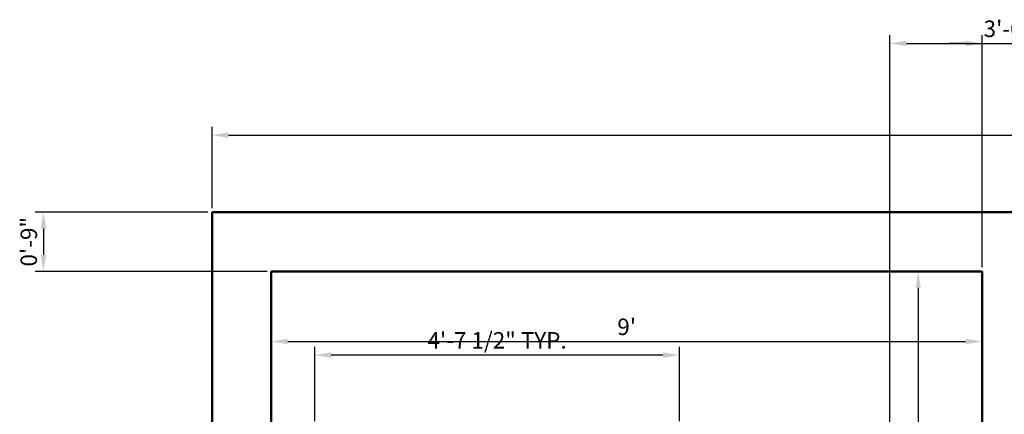
# Model space of a CAD drawing. Units: inches. Extents: x 2385 to 2740, y 1752 to 2305.
# Tile 10 of 15: x 2385 to 2535, y 2245 to 2305. Entities that reach past the tile are written whole.
import ezdxf

# ---------------------------------------------------------------- set-up
doc = ezdxf.new("R2010")
doc.units = ezdxf.units.IN
doc.layers.add('A-ANNO-DIMS', color=2, linetype='Continuous', lineweight=18)
doc.layers.add('A-WALL', color=7, linetype='Continuous', lineweight=50)
doc.styles.get("Standard").update_dxf_attribs({"font": 'arial.ttf'})
doc.dimstyles.new('Copy of ISO-25', dxfattribs={"dimtxt": 2.5, "dimasz": 2.5, "dimexe": 1.25, "dimexo": 0.625, "dimtad": 1, "dimdec": 1, "dimlunit": 4, "dimtxsty": 'Standard', "dimcen": 2.5, "dimadec": 0, "dimazin": 0, "dimtfac": 1, "dimtdec": 1, "dimtmove": 0, "dimatfit": 3, "dimfxl": 1, "dimarcsym": 0})

# ---------------------------------------------------------------- blocks, each defined once
blk = doc.blocks.new('*D6')
at = {"layer": 'A-ANNO-DIMS', "color": 0, "lineweight": -2, "transparency": 16777216}
for p, q in [((2423.25, 2266.34), (2423.25, 2255.07)), ((2531.25, 2266.34), (2531.25, 2255.07)), ((2425.75, 2256.32), (2528.75, 2256.32))]:
    blk.add_line(p, q, dxfattribs=at)
at = {"layer": 'A-ANNO-DIMS', "color": 0, "transparency": 16777216}
for points in [[(2425.75, 2256.74), (2425.75, 2255.91), (2423.25, 2256.32)], [(2528.75, 2256.74), (2528.75, 2255.91), (2531.25, 2256.32)]]:
    blk.add_solid(points, dxfattribs=at)
at = {"layer": 'Defpoints', "color": 0, "transparency": 16777216}
for p in [(2423.25, 2266.97), (2531.25, 2266.97), (2531.25, 2256.32)]:
    blk.add_point(p, dxfattribs=at)
at = {"layer": 'A-ANNO-DIMS', "color": 0, "transparency": 16777216, "insert": (2477.25, 2258.23), "char_height": 2.5, "attachment_point": 5}
blk.add_mtext("9'", dxfattribs=at)
blk = doc.blocks.new('*D7')
at = {"layer": 'A-ANNO-DIMS', "color": 0, "lineweight": -2, "transparency": 16777216}
for p, q in [((2530.62, 2266.97), (2520.29, 2266.97)), ((2521.54, 2264.47), (2521.54, 2143.47)), ((2530.62, 2140.97), (2520.29, 2140.97))]:
    blk.add_line(p, q, dxfattribs=at)
at = {"layer": 'A-ANNO-DIMS', "color": 0, "transparency": 16777216}
for points in [[(2521.12, 2264.47), (2521.95, 2264.47), (2521.54, 2266.97)], [(2521.12, 2143.47), (2521.95, 2143.47), (2521.54, 2140.97)]]:
    blk.add_solid(points, dxfattribs=at)
at = {"layer": 'Defpoints', "color": 0, "transparency": 16777216}
for p in [(2531.25, 2266.97), (2521.54, 2140.97), (2531.25, 2140.97)]:
    blk.add_point(p, dxfattribs=at)
at = {"layer": 'A-ANNO-DIMS', "color": 0, "transparency": 16777216, "insert": (2519.63, 2203.97), "char_height": 2.5, "attachment_point": 5, "rotation": 90}
blk.add_mtext('10\'-6"', dxfattribs=at)
blk = doc.blocks.new('*D24')
at = {"layer": 'A-ANNO-DIMS', "color": 0, "lineweight": -2, "transparency": 16777216}
for p, q in [((2414.25, 2276.59), (2414.25, 2288.91)), ((2712.25, 2276.59), (2712.25, 2288.91)), ((2416.75, 2287.66), (2709.75, 2287.66))]:
    blk.add_line(p, q, dxfattribs=at)
at = {"layer": 'A-ANNO-DIMS', "color": 0, "transparency": 16777216}
for points in [[(2416.75, 2288.08), (2416.75, 2287.25), (2414.25, 2287.66)], [(2709.75, 2288.08), (2709.75, 2287.25), (2712.25, 2287.66)]]:
    blk.add_solid(points, dxfattribs=at)
at = {"layer": 'Defpoints', "color": 0, "transparency": 16777216}
for p in [(2712.25, 2287.66), (2414.25, 2275.97), (2712.25, 2275.97)]:
    blk.add_point(p, dxfattribs=at)
at = {"layer": 'A-ANNO-DIMS', "color": 0, "transparency": 16777216, "insert": (2563.25, 2289.57), "char_height": 2.5, "attachment_point": 5}
blk.add_mtext('24\'-10"', dxfattribs=at)
blk = doc.blocks.new('*D27')
at = {"layer": 'A-ANNO-DIMS', "color": 0, "lineweight": -2, "transparency": 16777216}
for p, q in [((2429.86, 2244.24), (2429.86, 2255.5)), ((2485.26, 2244.24), (2485.26, 2255.5)), ((2482.76, 2254.25), (2432.36, 2254.25))]:
    blk.add_line(p, q, dxfattribs=at)
at = {"layer": 'A-ANNO-DIMS', "color": 0, "transparency": 16777216}
for points in [[(2432.36, 2254.67), (2432.36, 2253.84), (2429.86, 2254.25)], [(2482.76, 2254.67), (2482.76, 2253.84), (2485.26, 2254.25)]]:
    blk.add_solid(points, dxfattribs=at)
at = {"layer": 'Defpoints', "color": 0, "transparency": 16777216}
for p in [(2429.86, 2254.25), (2429.86, 2243.62), (2485.26, 2243.62)]:
    blk.add_point(p, dxfattribs=at)
at = {"layer": 'A-ANNO-DIMS', "color": 0, "transparency": 16777216, "insert": (2457.56, 2256.17), "char_height": 2.5, "attachment_point": 5}
blk.add_mtext('4\'-7 1/2" TYP.', dxfattribs=at)
blk = doc.blocks.new('*D39')
at = {"layer": 'A-ANNO-DIMS', "color": 0, "lineweight": -2, "transparency": 16777216}
for p, q in [((2531.25, 2267.59), (2531.25, 2302.84)), ((2537.25, 2267.59), (2537.25, 2302.84)), ((2528.75, 2301.59), (2526.25, 2301.59)), ((2531.25, 2301.59), (2537.25, 2301.59)), ((2539.75, 2301.59), (2550.14, 2301.59))]:
    blk.add_line(p, q, dxfattribs=at)
at = {"layer": 'A-ANNO-DIMS', "color": 0, "transparency": 16777216}
for points in [[(2528.75, 2302), (2528.75, 2301.17), (2531.25, 2301.59)], [(2539.75, 2302), (2539.75, 2301.17), (2537.25, 2301.59)]]:
    blk.add_solid(points, dxfattribs=at)
at = {"layer": 'Defpoints', "color": 0, "transparency": 16777216}
for p in [(2537.25, 2301.59), (2531.25, 2266.97), (2537.25, 2266.97)]:
    blk.add_point(p, dxfattribs=at)
at = {"layer": 'A-ANNO-DIMS', "color": 0, "transparency": 16777216, "insert": (2546.2, 2303.49), "char_height": 2.5, "attachment_point": 5}
blk.add_mtext('0\'-6"', dxfattribs=at)
blk = doc.blocks.new('*D40')
at = {"layer": 'A-ANNO-DIMS', "color": 0, "lineweight": -2, "transparency": 16777216}
for p, q in [((2413.62, 2275.97), (2387.38, 2275.97)), ((2388.63, 2273.47), (2388.63, 2269.47)), ((2422.62, 2266.97), (2387.38, 2266.97))]:
    blk.add_line(p, q, dxfattribs=at)
at = {"layer": 'A-ANNO-DIMS', "color": 0, "transparency": 16777216}
for points in [[(2388.21, 2273.47), (2389.05, 2273.47), (2388.63, 2275.97)], [(2388.21, 2269.47), (2389.05, 2269.47), (2388.63, 2266.97)]]:
    blk.add_solid(points, dxfattribs=at)
at = {"layer": 'Defpoints', "color": 0, "transparency": 16777216}
for p in [(2414.25, 2275.97), (2388.63, 2266.97), (2423.25, 2266.97)]:
    blk.add_point(p, dxfattribs=at)
at = {"layer": 'A-ANNO-DIMS', "color": 0, "transparency": 16777216, "insert": (2386.73, 2271.47), "char_height": 2.5, "attachment_point": 5, "rotation": 90}
blk.add_mtext('0\'-9"', dxfattribs=at)
blk = doc.blocks.new('*D48')
at = {"layer": 'A-ANNO-DIMS', "color": 0, "lineweight": -2, "transparency": 16777216}
for p, q in [((2517.25, 1916.59), (2517.25, 2302.84)), ((2553.25, 1916.59), (2553.25, 2302.84)), ((2519.75, 2301.59), (2550.75, 2301.59))]:
    blk.add_line(p, q, dxfattribs=at)
at = {"layer": 'A-ANNO-DIMS', "color": 0, "transparency": 16777216}
for points in [[(2519.75, 2302), (2519.75, 2301.17), (2517.25, 2301.59)], [(2550.75, 2302), (2550.75, 2301.17), (2553.25, 2301.59)]]:
    blk.add_solid(points, dxfattribs=at)
at = {"layer": 'Defpoints', "color": 0, "transparency": 16777216}
for p in [(2553.25, 2301.59), (2517.25, 1915.97), (2553.25, 1915.97)]:
    blk.add_point(p, dxfattribs=at)
at = {"layer": 'A-ANNO-DIMS', "color": 0, "transparency": 16777216, "insert": (2535.25, 2303.49), "char_height": 2.5, "attachment_point": 5}
blk.add_mtext('3\'-0"', dxfattribs=at)

msp = doc.modelspace()

# ---------------------------------------------------------------- linework, layer by layer
at = {"layer": 'A-WALL'}
for p, q in [((2414.25, 2275.97), (2694.25, 2275.97)), ((2414.25, 2266.97), (2414.25, 2275.97)), ((2414.25, 2275.97), (2712.25, 2275.97)), ((2414.25, 1924.97), (2414.25, 2266.97)), ((2531.25, 2266.97), (2423.25, 2266.97)), ((2423.25, 2266.97), (2423.25, 2146.97)), ((2531.25, 2266.97), (2423.25, 2266.97)), ((2531.25, 2146.97), (2531.25, 2266.97))]:
    msp.add_line(p, q, dxfattribs=at)

# ---------------------------------------------------------------- dimensions: what is measured, and where the dimension line sits
at = {"layer": 'A-ANNO-DIMS'}
for base, p1, p2, override, picture, middle in [((2553.25, 2301.59), (2517.25, 1915.97), (2553.25, 1915.97), {"dimdec": 1, "dimlfac": 1, "dimrnd": 0, "dimzin": 1, "dimdsep": 46, "dimlunit": 4, "dimfrac": 2}, '*D48', (2535.25, 2303.49)), ((2537.25, 2301.59), (2531.25, 2266.97), (2537.25, 2266.97), {"dimdec": 1, "dimlfac": 1, "dimrnd": 0, "dimzin": 1, "dimdsep": 46, "dimlunit": 4, "dimfrac": 2}, '*D39', (2546.2, 2303.49)), ((2712.25, 2287.66), (2414.25, 2275.97), (2712.25, 2275.97), {"dimclrd": 0, "dimclre": 0, "dimclrt": 0}, '*D24', (2563.25, 2289.57)), ((2531.25, 2256.32), (2423.25, 2266.97), (2531.25, 2266.97), {"dimclrd": 0, "dimclre": 0, "dimclrt": 0}, '*D6', (2477.25, 2258.23))]:
    dim = msp.add_linear_dim(base=base, p1=p1, p2=p2, dimstyle='Copy of ISO-25', override=override, dxfattribs=at)
    dim.commit()
    dim.dimension.update_dxf_attribs({"geometry": picture, "text_midpoint": middle})
for base, p1, p2, override, picture, middle in [((2388.63, 2266.97), (2414.25, 2275.97), (2423.25, 2266.97), {"dimdec": 1, "dimlfac": 1, "dimrnd": 0, "dimzin": 1, "dimdsep": 46, "dimlunit": 4, "dimfrac": 2}, '*D40', (2386.73, 2271.47)), ((2521.54, 2140.97), (2531.25, 2266.97), (2531.25, 2140.97), {"dimclrd": 0, "dimclre": 0, "dimclrt": 0}, '*D7', (2519.63, 2203.97))]:
    dim = msp.add_linear_dim(base=base, p1=p1, p2=p2, angle=90, dimstyle='Copy of ISO-25', override=override, dxfattribs=at)
    dim.commit()
    dim.dimension.update_dxf_attribs({"geometry": picture, "text_midpoint": middle})
dim = msp.add_linear_dim(base=(2429.86, 2254.25), p1=(2485.26, 2243.62), p2=(2429.86, 2243.62), angle=180, text='<> TYP.', dimstyle='Copy of ISO-25', override={"dimdec": 1, "dimlfac": 1, "dimrnd": 0, "dimzin": 1, "dimdsep": 46, "dimlunit": 4, "dimfrac": 2}, dxfattribs=at)
dim.commit()
dim.dimension.update_dxf_attribs({"geometry": '*D27', "text_midpoint": (2457.56, 2256.17)})

doc.saveas('drawing.dxf')
